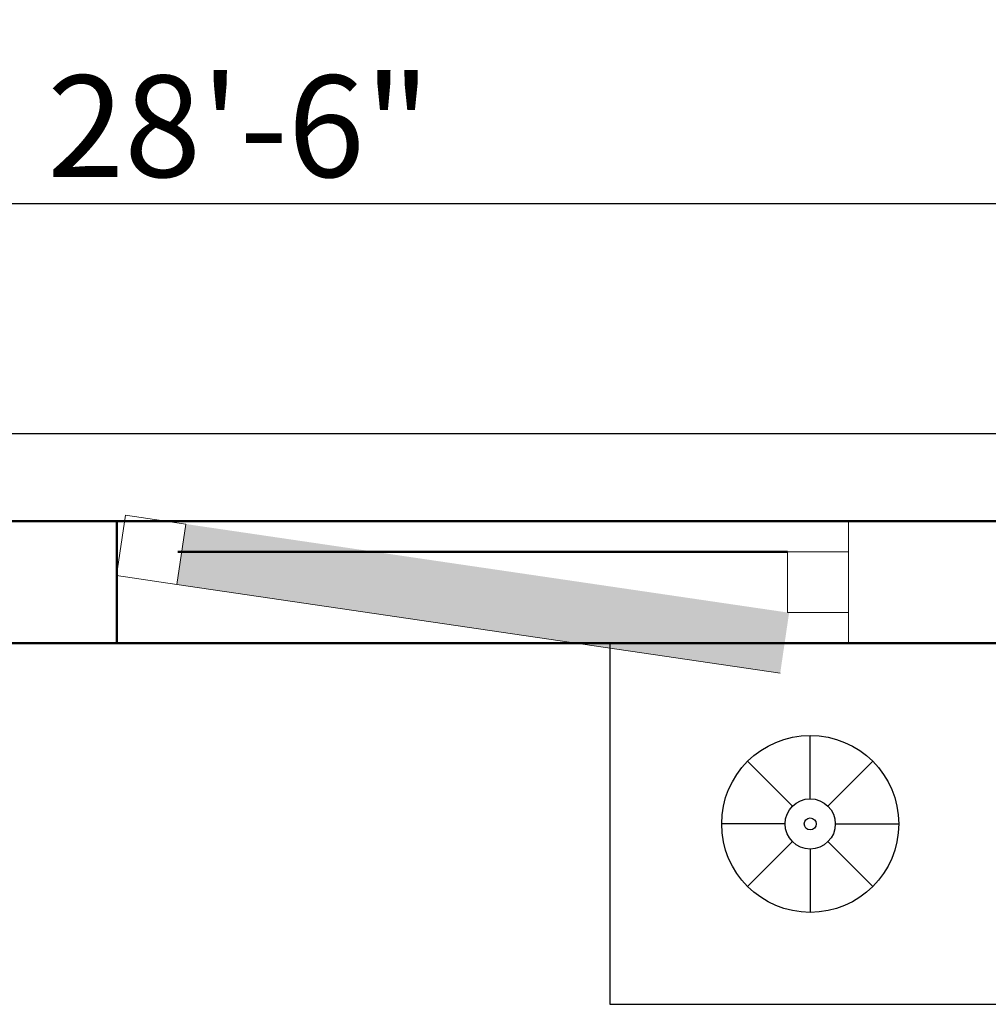
# Model space of a CAD drawing. Units: inches. Extents: x 3064 to 19385, y 846 to 15425.
# Tile 76 of 108: x 6629 to 6677, y 1964 to 2013. Entities that reach past the tile are written whole.
import ezdxf

# ---------------------------------------------------------------- set-up
doc = ezdxf.new("R2010")
doc.units = ezdxf.units.IN
for name, color, linetype, lineweight in [('A-ANNO-DIMS', 2, 'Continuous', 18), ('A-FLOR-FIXT', 9, 'Continuous', 18), ('A-GLAZ', 4, 'Continuous', 18), ('A-WALL', 7, 'Continuous', 50)]:
    doc.layers.add(name, color=color, linetype=linetype, lineweight=lineweight)
doc.layers.add('BLOCK', color=6, linetype='Continuous')
doc.styles.get("Standard").update_dxf_attribs({"font": 'arial.ttf'})
doc.dimstyles.new('ISO-25', dxfattribs={"dimtxt": 9, "dimasz": 2.5, "dimexe": 1.25, "dimexo": 0.625, "dimtad": 1, "dimdec": 1, "dimlunit": 3, "dimtxsty": 'Standard', "dimcen": 2.5, "dimadec": 0, "dimazin": 0, "dimtfac": 1, "dimtdec": 1, "dimtmove": 0, "dimatfit": 3, "dimfxl": 1, "dimarcsym": 0})

# ---------------------------------------------------------------- blocks, each defined once
blk = doc.blocks.new('A$C52E67D0D')
at = {"layer": 'BLOCK'}
for p, q in [((250.5, 1605.5), (250.5, 1684.7)), ((228.3, 1596.3), (172.3, 1652.3)), ((272.7, 1596.3), (328.7, 1652.3)), ((219.1, 1574.1), (139.9, 1574.1)), ((281.9, 1574.1), (361.1, 1574.1)), ((228.3, 1551.9), (172.3, 1495.9)), ((272.7, 1551.9), (328.7, 1495.9)), ((250.5, 1542.8), (250.5, 1463.5))]:
    blk.add_line(p, q, dxfattribs=at)
blk.add_lwpolyline([(501, 1348.6), (501, 1799.6), (0, 1799.6), (0, 1348.6)], close=True, dxfattribs=at)
for radius in [110.6, 31.4, 7.46]:
    blk.add_circle((250.5, 1574.1), radius, dxfattribs=at)
blk = doc.blocks.new('*D344')
at = {"layer": 'A-ANNO-DIMS', "color": 0, "lineweight": -2, "transparency": 16777216}
for p, q in [((6610.034, 1988.614), (6610.034, 1993.551)), ((6805.034, 1988.614), (6805.034, 1993.551)), ((6612.534, 1992.301), (6802.534, 1992.301))]:
    blk.add_line(p, q, dxfattribs=at)
at = {"layer": 'A-ANNO-DIMS', "color": 0, "transparency": 16777216}
for points in [[(6612.534, 1992.718), (6612.534, 1991.884), (6610.034, 1992.301)], [(6802.534, 1992.718), (6802.534, 1991.884), (6805.034, 1992.301)]]:
    blk.add_solid(points, dxfattribs=at)
at = {"layer": 'Defpoints', "color": 0, "transparency": 16777216}
for p in [(6805.034, 1992.301), (6610.034, 1987.989), (6805.034, 1987.989)]:
    blk.add_point(p, dxfattribs=at)
at = {"layer": 'A-ANNO-DIMS', "color": 0, "transparency": 16777216, "insert": (6707.534, 1995.481), "char_height": 5, "attachment_point": 5}
blk.add_mtext('16\'-3"', dxfattribs=at)
blk = doc.blocks.new('*D340')
at = {"layer": 'A-ANNO-DIMS', "color": 0, "lineweight": -2, "transparency": 16777216}
for p, q in [((6469.034, 1988.614), (6469.034, 2004.848)), ((6811.034, 1988.614), (6811.034, 2004.848)), ((6808.534, 2003.598), (6471.534, 2003.598))]:
    blk.add_line(p, q, dxfattribs=at)
at = {"layer": 'A-ANNO-DIMS', "color": 0, "transparency": 16777216}
for points in [[(6471.534, 2004.015), (6471.534, 2003.182), (6469.034, 2003.598)], [(6808.534, 2004.015), (6808.534, 2003.182), (6811.034, 2003.598)]]:
    blk.add_solid(points, dxfattribs=at)
at = {"layer": 'Defpoints', "color": 0, "transparency": 16777216}
for p in [(6469.034, 2003.598), (6469.034, 1987.989), (6811.034, 1987.989)]:
    blk.add_point(p, dxfattribs=at)
at = {"layer": 'A-ANNO-DIMS', "color": 0, "transparency": 16777216, "insert": (6640.034, 2006.776), "char_height": 5, "attachment_point": 5}
blk.add_mtext('28\'-6"', dxfattribs=at)
blk = doc.blocks.new('WIN-900-A')
h = blk.add_hatch(color=256)
h.dxf.hatch_style = 1
h.paths.add_polyline_path([(33, 0), (33, 3), (3, 3), (3, 0)])
blk.add_line((3, 0), (33, 0))
blk.add_lwpolyline([(3, 0), (0, 0), (0, 3), (3, 3)], close=True)
blk = doc.blocks.new('*D433')
at = {"layer": 'A-ANNO-DIMS', "color": 0, "lineweight": -2, "transparency": 16777216}
for p, q in [((6621.842, 1945.073), (6633.117, 2118.247)), ((6612.137, 1945.705), (6623.089, 1944.992)), ((6617.521, 1878.714), (6621.679, 1942.579)), ((6607.654, 1876.851), (6618.606, 1876.138))]:
    blk.add_line(p, q, dxfattribs=at)
at = {"layer": 'A-ANNO-DIMS', "color": 0, "transparency": 16777216}
for points in [[(6621.263, 1942.606), (6622.095, 1942.551), (6621.842, 1945.073)], [(6617.105, 1878.741), (6617.937, 1878.687), (6617.358, 1876.219)]]:
    blk.add_solid(points, dxfattribs=at)
at = {"layer": 'Defpoints', "color": 0, "transparency": 16777216}
for p in [(6611.513, 1945.746), (6621.842, 1945.073), (6607.03, 1876.892)]:
    blk.add_point(p, dxfattribs=at)
at = {"layer": 'A-ANNO-DIMS', "color": 0, "transparency": 16777216, "insert": (6622.29, 2033.251), "char_height": 9, "attachment_point": 5, "rotation": 86.2748}
blk.add_mtext('WINDOW W1900-A 5\'-9" TYP.', dxfattribs=at)

msp = doc.modelspace()

# ---------------------------------------------------------------- linework, layer by layer
at = {"layer": 'A-GLAZ'}
msp.add_line((6670.034, 1987.989), (6670.034, 1981.989), dxfattribs=at)
msp.add_lwpolyline([(6670.034, 1983.489), (6667.034, 1983.489), (6667.034, 1986.489), (6670.034, 1986.489)], close=True, dxfattribs=at)
at = {"layer": 'A-WALL'}
for p, q in [((6811.034, 1987.989), (6469.034, 1987.989)), ((6634.034, 1987.989), (6634.034, 1981.989)), ((6637.034, 1986.489), (6667.034, 1986.489)), ((6805.034, 1981.989), (6610.034, 1981.989))]:
    msp.add_line(p, q, dxfattribs=at)

# ---------------------------------------------------------------- block references
at = {"layer": 'A-FLOR-FIXT', "xscale": 0.039370099999992, "yscale": 0.039370099999992, "zscale": 0.039370099999992}
msp.add_blockref('A$C52E67D0D', (6658.282, 1911.123), dxfattribs=at)
at = {"layer": 'A-GLAZ', "rotation": 351.6350998303226}
msp.add_blockref('WIN-900-A', (6634.021, 1985.318), dxfattribs=at)

# ---------------------------------------------------------------- dimensions: what is measured, and where the dimension line sits
at = {"layer": 'A-ANNO-DIMS'}
dim = msp.add_linear_dim(base=(6621.842, 1945.073), p1=(6607.03, 1876.892), p2=(6611.513, 1945.746), angle=86.2748, text='WINDOW W1900-A <> TYP.', dimstyle='ISO-25', override={"dimdec": 1, "dimrnd": 0, "dimzin": 1, "dimlunit": 4, "dimfrac": 2}, dxfattribs=at)
dim.commit()
dim.dimension.update_dxf_attribs({"geometry": '*D433', "text_midpoint": (6622.29, 2033.251)})
for base, p1, p2, override, picture, middle in [((6469.034, 2003.598), (6811.034, 1987.989), (6469.034, 1987.989), {"dimtxt": 5, "dimclrd": 0, "dimclre": 0, "dimclrt": 0}, '*D340', (6640.034, 2006.776)), ((6805.034, 1992.301), (6610.034, 1987.989), (6805.034, 1987.989), {"dimtxt": 5, "dimclrd": 0, "dimclre": 0, "dimclrt": 0, "dimtmove": 1}, '*D344', (6707.534, 1995.481))]:
    dim = msp.add_linear_dim(base=base, p1=p1, p2=p2, dimstyle='ISO-25', override=override, dxfattribs=at)
    dim.commit()
    dim.dimension.update_dxf_attribs({"geometry": picture, "text_midpoint": middle})

doc.saveas('drawing.dxf')
